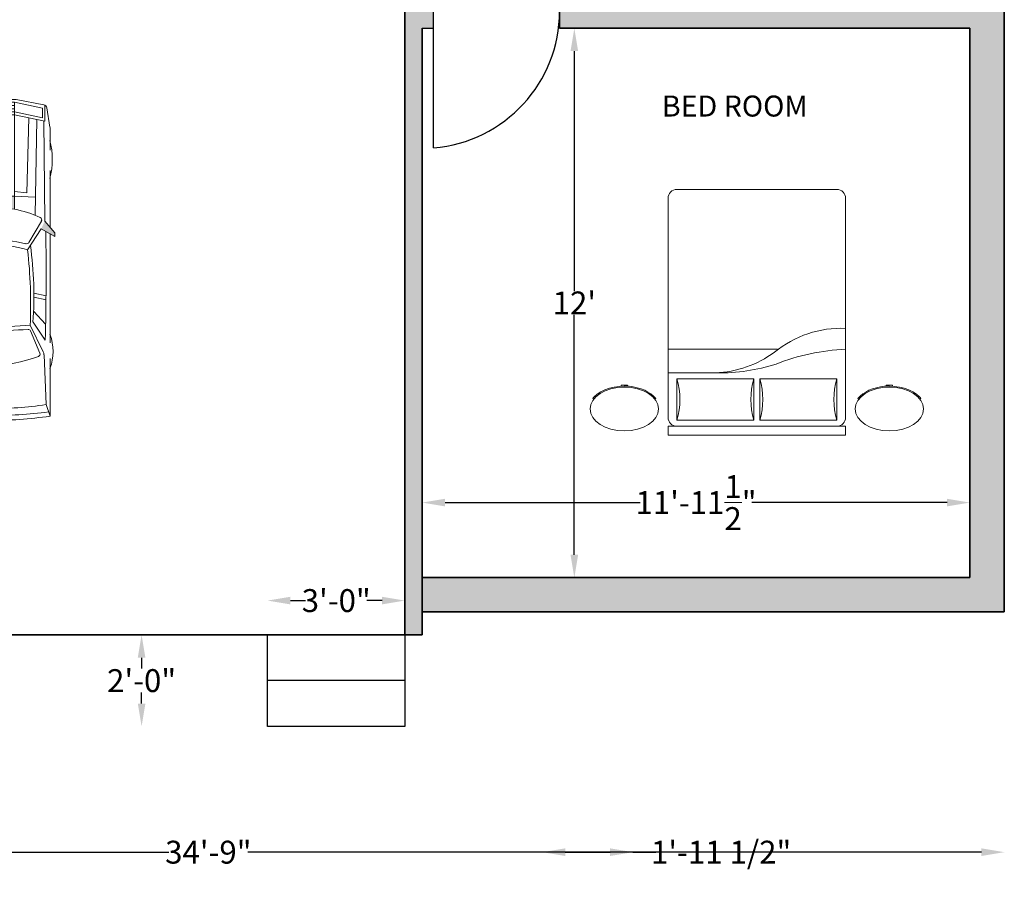
# Model space of a CAD drawing. Units: inches. Extents: x 2490 to 2996, y 1528 to 2269.
# Tile 2 of 4: x 2693 to 2951, y 1528 to 1755. Entities that reach past the tile are written whole.
import ezdxf

# ---------------------------------------------------------------- set-up
doc = ezdxf.new("R2010")
doc.units = ezdxf.units.IN
for name, color, linetype, lineweight in [('A-ANNO-DIMS', 2, 'Continuous', 18), ('A-DOOR', 4, 'Continuous', 25), ('A-EQPM-VEHL', 9, 'Continuous', 18), ('A-FLOR-STRS', 7, 'Continuous', 25), ('A-FURN', 8, 'Continuous', 18), ('A-WALL', 7, 'Continuous', 35)]:
    doc.layers.add(name, color=color, linetype=linetype, lineweight=lineweight)
doc.layers.add('A-AREA-IDEN', color=244, linetype='Continuous', lineweight=25, true_color=0x991b1e)
doc.layers.add('A-WALL-PATT', color=85, linetype='Continuous', lineweight=13, true_color=0x58ba48)
doc.styles.add('ATTR', font='romans.shx', dxfattribs={"width": 0.8, "height": 1.114828})
doc.styles.get("Standard").update_dxf_attribs({"font": 'arial.ttf'})
doc.dimstyles.get("Standard").update_dxf_attribs({"dimtxt": 6, "dimasz": 6, "dimexe": 0.18, "dimexo": 0.0625, "dimgap": 0.09, "dimtad": 0, "dimtih": 1, "dimtoh": 1, "dimdec": 4, "dimzin": 0, "dimdsep": 46, "dimlunit": 4, "dimtxsty": 'Standard', "dimcen": 0.09, "dimse1": 1, "dimse2": 1, "dimadec": 0, "dimazin": 0, "dimtfac": 1, "dimtdec": 4, "dimtofl": 0, "dimtmove": 0, "dimatfit": 3, "dimfxl": 1, "dimtolj": 1, "dimtzin": 0, "dimarcsym": 0})

# ---------------------------------------------------------------- blocks, each defined once
blk = doc.blocks.new('A$C682073C8')
for p, q in [((-2.694, 0.6), (-2.493, 0.633)), ((-2.251, 0.635), (-2.478, 0.635)), ((-1.445, 0.635), (-2.04, 0.635)), ((-1.51, 0.58), (-1.388, 0.684)), ((-1.428, 0.543), (-1.348, 0.684)), ((-1.388, 0.684), (-1.348, 0.684)), ((-0.237, 0.635), (-1.376, 0.635)), ((0.532, 0.635), (-0.072, 0.635)), ((0.532, 0.635), (0.411, 0.593)), ((-2.78, 0.282), (-2.724, 0.571)), ((-2.69, 0.555), (-2.752, 0.263)), ((-2.554, 0.581), (-2.72, 0.581)), ((-2.59, 0.555), (-2.69, 0.555)), ((-2.59, 0.555), (-2.652, 0.263)), ((-2.554, 0.581), (-2.622, 0.263)), ((-2.557, 0.57), (-1.51, 0.58)), ((-1.286, 0.414), (-1.508, 0.544)), ((-1.209, 0.401), (-1.428, 0.543)), ((-0.755, 0.467), (-0.727, 0.593)), ((-0.714, 0.467), (-0.686, 0.593)), ((-0.432, 0.589), (-0.565, 0.464)), ((-0.451, 0.457), (-0.263, 0.585)), ((-0.142, 0.564), (-0.42, 0.428)), ((-0.361, 0.431), (-0.128, 0.528)), ((0.411, 0.593), (-0.11, 0.572)), ((-1.805, 0.393), (-2.59, 0.413)), ((-1.57, 0.478), (-2.572, 0.496)), ((-1.771, 0.263), (-1.758, 0.481)), ((-1.818, 0.263), (-1.805, 0.393)), ((-2.781, 0), (-2.781, 0.273)), ((-2.752, 0.263), (-2.752, 0)), ((-1.633, 0.263), (-2.752, 0.263)), ((-2.718, 0.263), (-2.718, 0)), ((-2.685, 0.263), (-2.685, 0)), ((-2.652, 0.263), (-2.652, 0)), ((-2.622, 0.263), (-2.622, 0)), ((-1.771, 0.263), (-1.771, 0)), ((-1.633, 0.263), (-1.659, 0)), ((-2.652, 0.197), (-2.752, 0.197)), ((-2.652, 0.132), (-2.752, 0.132)), ((-2.781, 0), (-2.781, -0.273)), ((-2.652, 0.066), (-2.752, 0.066)), ((-2.652, 0), (-2.752, 0)), ((-2.752, -0.263), (-2.752, 0)), ((-2.718, -0.263), (-2.718, 0)), ((-2.685, -0.263), (-2.685, 0)), ((-2.652, -0.263), (-2.652, 0)), ((-2.622, -0.263), (-2.622, 0)), ((-1.771, -0.263), (-1.771, 0)), ((-1.659, 0), (-1.633, -0.263)), ((-2.652, -0.066), (-2.752, -0.066)), ((-2.652, -0.132), (-2.752, -0.132)), ((-2.652, -0.197), (-2.752, -0.197)), ((-2.78, -0.282), (-2.724, -0.571)), ((-1.633, -0.263), (-2.752, -0.263)), ((-2.69, -0.555), (-2.752, -0.263)), ((-2.59, -0.555), (-2.652, -0.263)), ((-2.554, -0.581), (-2.622, -0.263)), ((-1.818, -0.263), (-1.805, -0.393)), ((-1.771, -0.263), (-1.758, -0.481)), ((-1.805, -0.393), (-2.59, -0.413)), ((-1.209, -0.401), (-1.428, -0.543)), ((-1.57, -0.478), (-2.572, -0.496)), ((-1.286, -0.414), (-1.508, -0.544)), ((-0.755, -0.467), (-0.727, -0.593)), ((-0.714, -0.467), (-0.686, -0.593)), ((-0.432, -0.589), (-0.565, -0.464)), ((-0.451, -0.457), (-0.263, -0.585)), ((-0.142, -0.564), (-0.42, -0.428)), ((-0.361, -0.431), (-0.128, -0.528)), ((-2.554, -0.581), (-2.72, -0.581)), ((-2.694, -0.6), (-2.493, -0.633)), ((-2.59, -0.555), (-2.69, -0.555)), ((-2.557, -0.57), (-1.51, -0.58)), ((-1.51, -0.58), (-1.388, -0.684)), ((-1.428, -0.543), (-1.348, -0.684)), ((0.411, -0.593), (-0.11, -0.572)), ((0.532, -0.635), (0.411, -0.593)), ((-2.251, -0.635), (-2.478, -0.635)), ((-1.445, -0.635), (-2.04, -0.635)), ((-1.388, -0.684), (-1.348, -0.684)), ((-0.237, -0.635), (-1.376, -0.635)), ((0.532, -0.635), (-0.072, -0.635))]:
    blk.add_line(p, q)
for centre, radius, start, end in [((-2.478, 0.542), 0.0932, 90, 99.5555), ((-2.154, -0.189), 0.847, 76.4679, 103.5321), ((-0.146, 0.162), 0.505, 69.2613, 110.7387), ((-4.512, 0), 5.038, 360, 7.0662), ((-3.75, 0), 4.328, 360, 8.4328), ((-2.688, 0.564), 0.0366, 99.5555, 168.9219), ((-0.341, 0), 1.319, 156.2323, 168.4871), ((-1.522, 0.52), 0.0277, 59.6014, 156.2323), ((-0.97, -26.413), 27.007, 88.4985, 90.9138), ((-0.106, 0.49), 0.0817, 92.3222, 116.0777), ((-0.118, 0.504), 0.0264, 20.6689, 112.6283), ((-3.642, 0), 4.096, 360, 8.3245), ((-1.3, 0.39), 0.0277, 346.5017, 59.6014), ((-0.728, -3.189), 3.656, 85.6618, 98.2609), ((-0.642, -4.704), 5.136, 87.5218, 96.3432), ((-5.551, 0), 5.149, 360, 4.7655), ((-0.35, 0.407), 0.0264, 112.6283, 183.982), ((-1.453, 0), 1.453, 360, 20.6689), ((0.324, 0), 1.642, 166.5017, 180), ((0.222, 0), 1.487, 164.3473, 180), ((-6.195, 0), 5.833, 360, 3.982), ((-2.736, 0.273), 0.045, 168.9219, 180), ((0.324, 0), 1.642, 180, 193.4983), ((0.222, 0), 1.487, 180, 195.6527), ((-5.551, 0), 5.149, 355.2345, 360), ((-6.195, 0), 5.833, 356.018, 360), ((-1.453, 0), 1.453, 339.3311, 360), ((-3.642, 0), 4.096, 351.6755, 360), ((-4.512, 0), 5.038, 352.9338, 360), ((-3.75, 0), 4.328, 351.5672, 360), ((-2.736, -0.273), 0.045, 180, 191.0781), ((-0.341, 0), 1.319, 191.5129, 203.7677), ((-1.3, -0.39), 0.0277, 300.3986, 13.4983), ((-0.642, 4.704), 5.136, 263.6568, 272.4781), ((-0.35, -0.407), 0.0264, 176.018, 247.3717), ((-0.728, 3.189), 3.656, 261.7391, 274.3382), ((-0.118, -0.504), 0.0264, 247.3717, 339.3311), ((-2.688, -0.564), 0.0366, 191.0781, 260.4445), ((-1.522, -0.52), 0.0277, 203.7677, 300.3986), ((-0.97, 26.413), 27.007, 269.0862, 271.5015), ((-0.106, -0.49), 0.0817, 243.9223, 267.6778), ((-2.478, -0.542), 0.0932, 260.4445, 270), ((-2.154, 0.189), 0.847, 256.4679, 283.5321), ((-0.146, -0.162), 0.505, 249.2613, 290.7387)]:
    blk.add_arc(centre, radius, start, end)
for points in [[(-1.428, 0.543), (-1.51, 0.58), (-1.348, 0.684), (-1.388, 0.684)], [(-1.633, 0.263), (-1.659, 0), (-1.771, 0.263), (-1.771, -0.263)], [(-1.659, 0), (-1.633, -0.263), (-1.771, -0.263)], [(-1.428, -0.543), (-1.51, -0.58), (-1.348, -0.684), (-1.388, -0.684)]]:
    blk.add_solid(points)
at = {"style": 'ATTR', "width": 0.8, "flags": 9}
blk.add_attdef('ESTCODE', (-2.781, 0), '', height=0.00071, rotation=180, dxfattribs=at)
blk = doc.blocks.new('*D20')
at = {"layer": 'A-ANNO-DIMS', "color": 0, "lineweight": -2, "transparency": 16777216}
for p, q in [((2838.65, 1747.13), (2838.65, 1684.23)), ((2838.65, 1615.13), (2838.65, 1678.03))]:
    blk.add_line(p, q, dxfattribs=at)
at = {"layer": 'A-ANNO-DIMS', "color": 0, "transparency": 16777216}
for points in [[(2837.65, 1747.13), (2839.65, 1747.13), (2838.65, 1753.13)], [(2837.65, 1615.13), (2839.65, 1615.13), (2838.65, 1609.13)]]:
    blk.add_solid(points, dxfattribs=at)
at = {"layer": 'Defpoints', "color": 0, "transparency": 16777216}
for p in [(2942.28, 1753.13), (2838.65, 1609.13), (2942.28, 1609.13)]:
    blk.add_point(p, dxfattribs=at)
at = {"layer": 'A-ANNO-DIMS', "color": 0, "transparency": 16777216, "insert": (2838.65, 1681.13), "char_height": 6, "attachment_point": 5}
blk.add_mtext("\\A1;12'", dxfattribs=at)
blk = doc.blocks.new('*D21')
at = {"layer": 'A-ANNO-DIMS', "color": 0, "lineweight": -2, "transparency": 16777216}
for p, q in [((2804.78, 1628.8), (2855.9, 1628.8)), ((2936.28, 1628.8), (2885.16, 1628.8))]:
    blk.add_line(p, q, dxfattribs=at)
at = {"layer": 'A-ANNO-DIMS', "color": 0, "transparency": 16777216}
for points in [[(2804.78, 1629.8), (2804.78, 1627.8), (2798.78, 1628.8)], [(2936.28, 1629.8), (2936.28, 1627.8), (2942.28, 1628.8)]]:
    blk.add_solid(points, dxfattribs=at)
at = {"layer": 'Defpoints', "color": 0, "transparency": 16777216}
for p in [(2942.28, 1628.8), (2798.78, 1609.13), (2942.28, 1609.13)]:
    blk.add_point(p, dxfattribs=at)
at = {"layer": 'A-ANNO-DIMS', "color": 0, "transparency": 16777216, "insert": (2870.53, 1628.8), "char_height": 6, "attachment_point": 5}
blk.add_mtext('\\A1;11\'-11{\\H1x;\\S1/2;}"', dxfattribs=at)
blk = doc.blocks.new('BED-WITH-NIGHTSTANDS')
for p, q in [((20.41, 64.37), (66.94, 64.37)), ((20.41, 62.04), (20.41, 64.37)), ((20.41, 62.04), (66.94, 62.04)), ((66.94, 62.04), (66.94, 64.37)), ((20.41, 2.33), (20.41, 59.72)), ((22.74, 60.49), (22.74, 49.63)), ((42.9, 60.49), (22.74, 60.49)), ((42.9, 49.63), (42.9, 60.49)), ((64.61, 60.49), (44.45, 60.49)), ((44.45, 60.49), (44.45, 49.63)), ((64.61, 49.63), (64.61, 60.49)), ((66.94, 59.72), (66.94, 2.33)), ((0.95, 54.97), (0.72, 54.79)), ((16.97, 54.97), (17.2, 54.79)), ((70.38, 54.97), (70.15, 54.79)), ((86.4, 54.97), (86.63, 54.79)), ((22.74, 49.63), (42.9, 49.63)), ((44.45, 49.63), (64.61, 49.63)), ((54.15, 48.08), (66.94, 48.08)), ((38.25, 41.88), (66.94, 41.88)), ((64.61, 0), (22.74, 0))]:
    blk.add_line(p, q)
for points in [[(9.82, 51.55), (9.82, 51.29), (8.1, 51.29), (8.1, 51.56)], [(77.53, 51.55), (77.53, 51.29), (79.25, 51.29), (79.25, 51.56)]]:
    blk.add_lwpolyline(points)
for centre, radius, start, end in [((22.74, 59.72), 2.33, 90, 180), ((64.61, 59.72), 2.33, 0, 90), ((4.12, 55.06), 19.39, 343.7398, 16.2602), ((61.51, 55.06), 19.39, 163.7398, 196.2602), ((25.84, 55.06), 19.39, 343.7398, 16.2602), ((83.23, 55.06), 19.39, 163.7398, 196.2602), ((53.52, -0.58), 48.67, 89.2582, 107.8034), ((55.8, 19.6), 28.51, 92.5398, 126.0403), ((17.8, 98.89), 57.07, 272.616, 291.4069), ((21.57, 63.79), 27.41, 267.5673, 309.5461), ((22.74, 2.33), 2.33, 180, 270), ((64.61, 2.33), 2.33, 270, 0)]:
    blk.add_arc(centre, radius, start, end)
blk.add_ellipse((8.96, 57.54), major_axis=(-8.96, 0), ratio=0.638095)
at = {"extrusion": (0, 0, -1)}
blk.add_ellipse((78.39, 57.54), major_axis=(8.96, 0), ratio=0.638095, dxfattribs=at)
for points in [[(0.72, 54.79), (0.84, 54.64), (0.96, 54.5), (3, 52.37), (6.73, 51.27), (13.16, 51.84), (15.82, 53.08), (17.2, 54.8)], [(86.63, 54.79), (86.51, 54.64), (86.39, 54.5), (84.35, 52.37), (80.63, 51.27), (74.19, 51.84), (71.53, 53.08), (70.15, 54.8)]]:
    blk.add_open_spline(points, degree=3, knots=[0.464624, 0.464624, 0.464624, 0.464624, 0.54806, 0.54806, 1.710779, 1.710779, 2.676847, 2.676847, 2.676847, 2.676847])
blk = doc.blocks.new('*D46')
at = {"layer": 'A-ANNO-DIMS', "color": 0, "lineweight": -2, "transparency": 16777216}
for p, q in [((2540.28, 1537.16), (2732.39, 1537.16)), ((2945.28, 1537.16), (2753.17, 1537.16))]:
    blk.add_line(p, q, dxfattribs=at)
at = {"layer": 'A-ANNO-DIMS', "color": 0, "transparency": 16777216}
for points in [[(2540.28, 1538.16), (2540.28, 1536.16), (2534.28, 1537.16)], [(2945.28, 1538.16), (2945.28, 1536.16), (2951.28, 1537.16)]]:
    blk.add_solid(points, dxfattribs=at)
at = {"layer": 'Defpoints', "color": 0, "transparency": 16777216}
for p in [(2951.28, 1600.13), (2534.28, 1594.13), (2951.28, 1537.16)]:
    blk.add_point(p, dxfattribs=at)
at = {"layer": 'A-ANNO-DIMS', "color": 0, "transparency": 16777216, "insert": (2742.78, 1537.16), "char_height": 6, "attachment_point": 5}
blk.add_mtext('\\A1;34\'-9"', dxfattribs=at)
blk = doc.blocks.new('*D47')
at = {"layer": 'A-ANNO-DIMS', "color": 0, "lineweight": -2, "transparency": 16777216}
for p, q in [((2501.3, 2221.13), (2501.3, 1901.79)), ((2501.3, 1576.13), (2501.3, 1895.48))]:
    blk.add_line(p, q, dxfattribs=at)
at = {"layer": 'A-ANNO-DIMS', "color": 0, "transparency": 16777216}
for points in [[(2500.3, 2221.13), (2502.3, 2221.13), (2501.3, 2227.13)], [(2500.3, 1576.13), (2502.3, 1576.13), (2501.3, 1570.13)]]:
    blk.add_solid(points, dxfattribs=at)
at = {"layer": 'Defpoints', "color": 0, "transparency": 16777216}
for p in [(2501.3, 2227.13), (2534.28, 2227.13), (2758.28, 1570.13)]:
    blk.add_point(p, dxfattribs=at)
at = {"layer": 'A-ANNO-DIMS', "color": 0, "transparency": 16777216, "insert": (2501.3, 1898.63), "char_height": 6, "attachment_point": 5}
blk.add_mtext('\\A1;54\'-9"', dxfattribs=at)
blk = doc.blocks.new('*D48')
at = {"layer": 'A-ANNO-DIMS', "color": 0, "lineweight": -2, "transparency": 16777216}
for p, q in [((2764.28, 1603.11), (2768.22, 1603.11)), ((2788.28, 1603.11), (2784.34, 1603.11))]:
    blk.add_line(p, q, dxfattribs=at)
at = {"layer": 'A-ANNO-DIMS', "color": 0, "transparency": 16777216}
for points in [[(2764.28, 1604.11), (2764.28, 1602.11), (2758.28, 1603.11)], [(2788.28, 1604.11), (2788.28, 1602.11), (2794.28, 1603.11)]]:
    blk.add_solid(points, dxfattribs=at)
at = {"layer": 'Defpoints', "color": 0, "transparency": 16777216}
for p in [(2794.28, 1603.11), (2758.28, 1570.13), (2794.28, 1570.13)]:
    blk.add_point(p, dxfattribs=at)
at = {"layer": 'A-ANNO-DIMS', "color": 0, "transparency": 16777216, "insert": (2776.28, 1603.11), "char_height": 6, "attachment_point": 5}
blk.add_mtext('\\A1;3\'-0"', dxfattribs=at)
blk = doc.blocks.new('*D49')
at = {"layer": 'A-ANNO-DIMS', "color": 0, "lineweight": -2, "transparency": 16777216}
for p, q in [((2725.3, 1588.13), (2725.3, 1585.29)), ((2725.3, 1576.13), (2725.3, 1578.98))]:
    blk.add_line(p, q, dxfattribs=at)
at = {"layer": 'A-ANNO-DIMS', "color": 0, "transparency": 16777216}
for points in [[(2724.3, 1588.13), (2726.3, 1588.13), (2725.3, 1594.13)], [(2724.3, 1576.13), (2726.3, 1576.13), (2725.3, 1570.13)]]:
    blk.add_solid(points, dxfattribs=at)
at = {"layer": 'Defpoints', "color": 0, "transparency": 16777216}
for p in [(2725.3, 1594.13), (2758.28, 1594.13), (2758.28, 1570.13)]:
    blk.add_point(p, dxfattribs=at)
at = {"layer": 'A-ANNO-DIMS', "color": 0, "transparency": 16777216, "insert": (2725.3, 1582.13), "char_height": 6, "attachment_point": 5}
blk.add_mtext('\\A1;2\'-0"', dxfattribs=at)
blk = doc.blocks.new('*D60')
at = {"layer": 'A-ANNO-DIMS', "color": 0, "lineweight": -2, "transparency": 16777216}
for p, q in [((2836.26, 1537.16), (2848, 1537.16)), ((2854, 1537.16), (2860, 1537.16))]:
    blk.add_line(p, q, dxfattribs=at)
at = {"layer": 'A-ANNO-DIMS', "color": 0, "transparency": 16777216}
for points in [[(2836.26, 1538.16), (2836.26, 1536.16), (2830.26, 1537.16)], [(2848, 1538.16), (2848, 1536.16), (2854, 1537.16)]]:
    blk.add_solid(points, dxfattribs=at)
at = {"layer": 'Defpoints', "color": 0, "transparency": 16777216}
for p in [(2830.26, 1968.5), (2854, 1968.5), (2854, 1537.16)]:
    blk.add_point(p, dxfattribs=at)
at = {"layer": 'A-ANNO-DIMS', "color": 0, "transparency": 16777216, "insert": (2877.11, 1537.16), "char_height": 6, "attachment_point": 5}
blk.add_mtext('\\A1;1\'-11 1/2"', dxfattribs=at)

msp = doc.modelspace()

# ---------------------------------------------------------------- hatches: boundary and pattern name
at = {"layer": 'A-WALL-PATT'}
h = msp.add_hatch(color=256, dxfattribs=at)
h.dxf.hatch_style = 1
h.paths.add_polyline_path([(2951.27862, 2227.13248), (2534.27862, 2227.13248), (2534.27862, 1594.13248), (2543.27862, 1594.13248), (2543.27862, 1776.13248), (2543.27862, 1780.63248), (2543.27862, 1788.13248), (2639.77862, 1788.13248), (2722.27862, 1788.13248), (2722.27862, 1792.63248), (2639.77862, 1792.63248), (2543.27862, 1792.63248), (2543.27862, 1822.63248), (2543.27862, 1876.63248), (2639.77862, 1876.63248), (2651.27862, 1876.63248), (2651.27862, 1881.13248), (2639.77862, 1881.13248), (2639.77862, 1884.13248), (2635.27862, 1884.13248), (2635.27862, 1881.13248), (2603.77862, 1881.13248), (2543.27862, 1881.13248), (2543.27862, 1977.13248), (2635.27862, 1977.13248), (2635.27862, 1917.13248), (2639.77862, 1917.13248), (2639.77862, 2057.63248), (2651.27862, 2057.63248), (2651.27862, 2062.13248), (2635.27862, 2062.13248), (2635.27862, 2057.63248), (2635.27862, 1981.63248), (2543.27862, 1981.63248), (2543.27862, 2057.63248), (2605.27862, 2057.63248), (2605.27862, 2062.13248), (2543.27862, 2062.13248), (2543.27862, 2218.13248), (2687.27862, 2218.13248), (2687.27862, 2062.13248), (2684.27862, 2062.13248), (2684.27862, 2057.63248), (2687.27862, 2057.63248), (2691.77862, 2057.63248), (2694.77862, 2057.63248), (2694.77862, 2062.13248), (2691.77862, 2062.13248), (2691.77862, 2093.63248), (2691.77862, 2218.13248), (2823.77862, 2218.13248), (2823.77862, 2062.13248), (2727.77862, 2062.13248), (2727.77862, 2057.63248), (2828.27862, 2057.63248), (2831.27862, 2057.63248), (2831.27862, 2062.13248), (2828.27862, 2062.13248), (2828.27862, 2093.63248), (2828.27862, 2218.13248), (2942.27862, 2218.13248), (2942.27862, 2062.13248), (2864.27862, 2062.13248), (2864.27862, 2057.63248), (2942.27862, 2057.63248), (2942.27862, 1757.63248), (2834.77862, 1757.63248), (2834.77862, 1753.13248), (2942.27862, 1753.13248), (2942.27862, 1609.13248), (2798.77862, 1609.13248), (2798.77862, 1600.13248), (2951.27862, 1600.13248)])
h.paths.add_polyline_path([(2798.77862, 1753.13248), (2801.77862, 1753.13248), (2801.77862, 1757.63248), (2798.77862, 1757.63248), (2798.77862, 1780.63248), (2798.77862, 1792.63248), (2794.27862, 1792.63248), (2794.27862, 1788.13248), (2794.27862, 1776.13248), (2794.27862, 1757.63248), (2794.27862, 1594.13248), (2798.77862, 1594.13248)], flags=17)

# ---------------------------------------------------------------- linework, layer by layer
at = {"layer": 'A-DOOR'}
for p, q in [((2801.77862, 1721.7577), (2801.77862, 1757.63248)), ((2798.77862, 1721.63248), (2798.77862, 1753.13248)), ((2798.77862, 1753.13248), (2801.77862, 1753.13248))]:
    msp.add_line(p, q, dxfattribs=at)
msp.add_arc((2798.77862, 1757.63248), 36, 274.7801918, 0, dxfattribs=at)
at = {"layer": 'A-FLOR-STRS'}
for p, q in [((2758.27862, 1582.13248), (2758.27862, 1594.13248)), ((2794.27862, 1594.13248), (2794.27862, 1582.13248)), ((2794.27862, 1582.13248), (2758.27862, 1582.13248)), ((2758.27862, 1570.13248), (2758.27862, 1582.13248)), ((2794.27862, 1582.13248), (2794.27862, 1570.13248)), ((2794.27862, 1570.13248), (2758.27862, 1570.13248))]:
    msp.add_line(p, q, dxfattribs=at)
at = {"layer": 'A-WALL'}
for p, q in [((2951.27862, 2227.13248), (2951.27862, 1600.13248)), ((2794.27862, 1757.63248), (2794.27862, 1594.13248)), ((2834.77862, 1757.63248), (2834.77862, 1753.13248)), ((2798.77862, 1753.13248), (2798.77862, 1594.13248)), ((2834.77862, 1753.13248), (2942.27862, 1753.13248)), ((2942.27862, 1753.13248), (2942.27862, 1609.13248)), ((2798.77862, 1609.13248), (2942.27862, 1609.13248)), ((2798.77862, 1600.13248), (2951.27862, 1600.13248)), ((2798.77862, 1594.13248), (2534.27862, 1594.13248))]:
    msp.add_line(p, q, dxfattribs=at)

# ---------------------------------------------------------------- block references
at = {"layer": 'A-EQPM-VEHL', "xscale": 25.05891406784298, "yscale": 25.05891406784298, "zscale": 25.05891406784298, "rotation": 270}
msp.add_blockref('A$C682073C8', (2685.40516, 1664.76968), dxfattribs=at)
at = {"layer": 'A-FURN', "rotation": 180}
msp.add_blockref('BED-WITH-NIGHTSTANDS', (2930.13041, 1710.87267), dxfattribs=at)

# ---------------------------------------------------------------- texts
at = {"layer": 'A-AREA-IDEN', "insert": (2861.57387, 1735.49489), "char_height": 5.501423, "attachment_point": 1}
msp.add_mtext_dynamic_manual_height_columns('BED ROOM ', width=200.8472283, gutter_width=27.50711, heights=[0], dxfattribs=at)

# ---------------------------------------------------------------- dimensions: what is measured, and where the dimension line sits
at = {"layer": 'A-ANNO-DIMS'}
for base, p1, p2, override, picture, middle in [((2501.30362, 2227.13248), (2758.27862, 1570.13248), (2534.27862, 2227.13248), {"dimdec": 1, "dimlfac": 1, "dimrnd": 0, "dimzin": 1, "dimdsep": 46, "dimlunit": 4, "dimfrac": 2}, '*D47', (2501.30362, 1898.63248)), ((2838.65434, 1609.13248), (2942.27862, 1753.13248), (2942.27862, 1609.13248), {"dimclrd": 0, "dimclre": 0, "dimclrt": 0}, '*D20', (2838.65434, 1681.13248)), ((2725.30362, 1594.13248), (2758.27862, 1570.13248), (2758.27862, 1594.13248), {"dimdec": 1, "dimlfac": 1, "dimrnd": 0, "dimzin": 1, "dimdsep": 46, "dimlunit": 4, "dimfrac": 2}, '*D49', (2725.30362, 1582.13248))]:
    dim = msp.add_linear_dim(base=base, p1=p1, p2=p2, angle=90, dimstyle='Standard', override=override, dxfattribs=at)
    dim.commit()
    dim.dimension.update_dxf_attribs({"geometry": picture, "text_midpoint": middle})
for base, p1, p2, override, picture, middle in [((2854.00162, 1537.15748), (2830.26433, 1968.49695), (2854.00162, 1968.49695), {"dimdec": 1, "dimlfac": 1, "dimrnd": 0, "dimzin": 1, "dimdsep": 46, "dimlunit": 4, "dimfrac": 2}, '*D60', (2877.10527, 1537.15748)), ((2942.27862, 1628.80089), (2798.77862, 1609.13248), (2942.27862, 1609.13248), {"dimclrd": 0, "dimclre": 0, "dimclrt": 0}, '*D21', (2870.52862, 1628.80089)), ((2794.27862, 1603.10748), (2758.27862, 1570.13248), (2794.27862, 1570.13248), {"dimdec": 1, "dimlfac": 1, "dimrnd": 0, "dimzin": 1, "dimdsep": 46, "dimlunit": 4, "dimfrac": 2}, '*D48', (2776.27862, 1603.10748)), ((2951.27862, 1537.15748), (2534.27862, 1594.13248), (2951.27862, 1600.13248), {"dimdec": 1, "dimlfac": 1, "dimrnd": 0, "dimzin": 1, "dimdsep": 46, "dimlunit": 4, "dimfrac": 2}, '*D46', (2742.77862, 1537.15748))]:
    dim = msp.add_linear_dim(base=base, p1=p1, p2=p2, dimstyle='Standard', override=override, dxfattribs=at)
    dim.commit()
    dim.dimension.update_dxf_attribs({"geometry": picture, "text_midpoint": middle})

doc.saveas('drawing.dxf')
